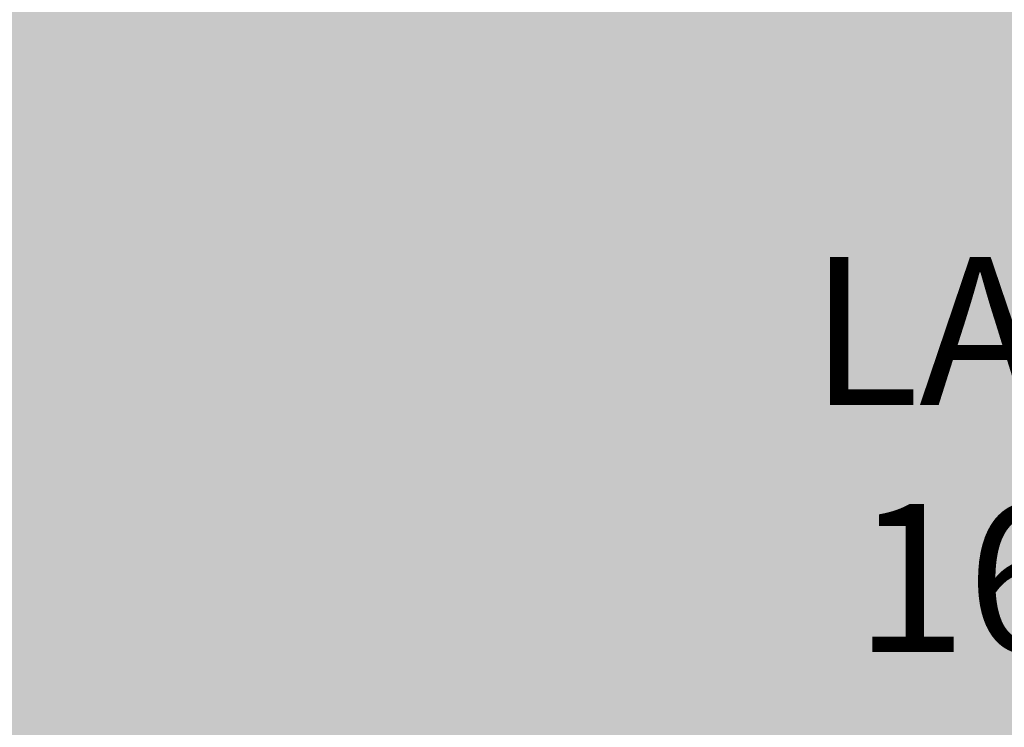
# Model space of a CAD drawing. Units: inches. Extents: x 84 to 1044, y -280 to 906.
# Tile 90 of 105: x 733 to 779, y 445 to 479. Entities that reach past the tile are written whole.
import ezdxf

# ---------------------------------------------------------------- set-up
doc = ezdxf.new("R2010")
doc.units = ezdxf.units.IN
doc.layers.add('A-ANNO-DIMS', color=2, linetype='Continuous', lineweight=18)
doc.layers.add('A-AREA-IDEN', color=7, linetype='Continuous', lineweight=13)
doc.layers.add('L-PLNT-PATT', color=9, linetype='Continuous', lineweight=9, true_color=0xafd9aa)
doc.styles.add('1-100DIM', font='txt', dxfattribs={"height": 0.3})
doc.styles.get("Standard").update_dxf_attribs({"font": 'arial.ttf'})
doc.dimstyles.get("Standard").update_dxf_attribs({"dimtxt": 0.18, "dimasz": 0.18, "dimexe": 0.18, "dimexo": 0.0625, "dimgap": 0.09, "dimtad": 0, "dimtih": 1, "dimtoh": 1, "dimdec": 4, "dimzin": 0, "dimdsep": 46, "dimtxsty": 'Standard', "dimcen": 0.09, "dimadec": 0, "dimazin": 0, "dimtfac": 1, "dimtdec": 4, "dimtofl": 0, "dimtmove": 0, "dimatfit": 3, "dimfxl": 1, "dimtolj": 1, "dimtzin": 0, "dimarcsym": 0})

# ---------------------------------------------------------------- blocks, each defined once
blk = doc.blocks.new('*D62')
at = {"layer": 'A-ANNO-DIMS', "color": 0, "lineweight": -2, "transparency": 16777216}
for p, q in [((203.179, 709.183), (203.179, 905.9)), ((203.359, 905.72), (549.232, 905.72)), ((895.894, 905.72), (550.021, 905.72)), ((896.074, 400.183), (896.074, 905.9))]:
    blk.add_line(p, q, dxfattribs=at)
at = {"layer": 'A-ANNO-DIMS', "color": 0, "transparency": 16777216}
for points in [[(203.359, 905.75), (203.359, 905.69), (203.179, 905.72)], [(895.894, 905.75), (895.894, 905.69), (896.074, 905.72)]]:
    blk.add_solid(points, dxfattribs=at)
at = {"layer": 'Defpoints', "color": 0, "transparency": 16777216}
for p in [(896.074, 905.72), (203.179, 709.12), (896.074, 400.12)]:
    blk.add_point(p, dxfattribs=at)
at = {"layer": 'A-ANNO-DIMS', "color": 0, "transparency": 16777216, "insert": (549.627, 905.72), "char_height": 0.18, "attachment_point": 5}
blk.add_mtext('\\A1;692.9', dxfattribs=at)

msp = doc.modelspace()

# ---------------------------------------------------------------- hatches: boundary and pattern name
at = {"layer": 'L-PLNT-PATT', "transparency": 33554597}
h = msp.add_hatch(color=256, dxfattribs=at)
h.dxf.hatch_style = 1
h.paths.add_polyline_path([(896.074, 511.12), (704.074, 511.12), (704.074, 491.62), (704.074, 419.62), (704.074, 400.12), (833.074, 400.12), (896.074, 400.12)])

# ---------------------------------------------------------------- texts
at = {"layer": 'A-AREA-IDEN', "insert": (769.898, 467.716), "char_height": 7, "attachment_point": 1, "style": '1-100DIM'}
msp.add_mtext_dynamic_manual_height_columns("{\\f@Malgun Gothic|b0|i0|c0|p34;LANDSCAPE\\P 16'0''X9'0''}", width=58.97918, gutter_width=15.851, heights=[0], dxfattribs=at)

# ---------------------------------------------------------------- dimensions: what is measured, and where the dimension line sits
at = {"layer": 'A-ANNO-DIMS'}
dim = msp.add_linear_dim(base=(896.074, 905.72), p1=(203.179, 709.12), p2=(896.074, 400.12), dimstyle='Standard', override={"dimdec": 1, "dimlfac": 1, "dimrnd": 0, "dimzin": 0, "dimdsep": 46, "dimlunit": 2}, dxfattribs=at)
dim.commit()
dim.dimension.update_dxf_attribs({"geometry": '*D62', "text_midpoint": (549.627, 905.72)})

doc.saveas('drawing.dxf')
